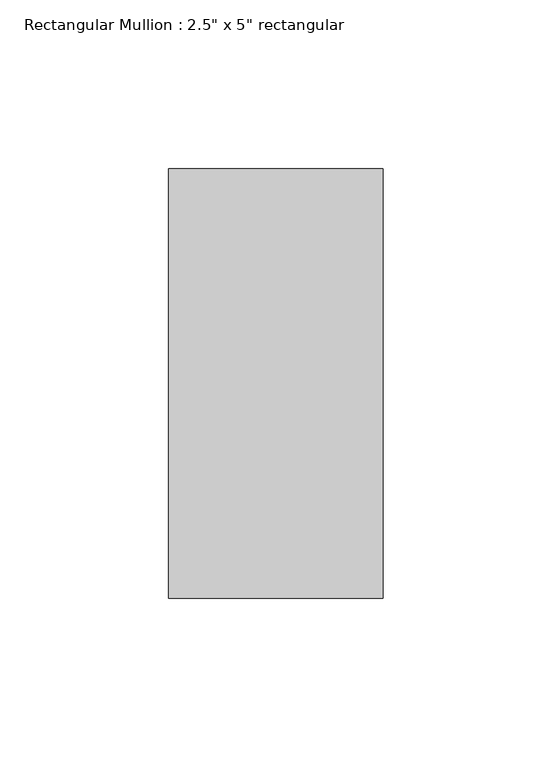
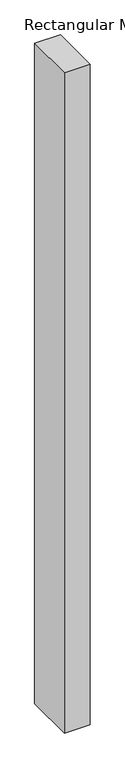
"""IFC4 building model written with IfcOpenShell, lengths in millimetres: member geometry."""

from ifc_helpers import new_model, si_unit, frame, origin, place, context, project, spatial, polyline, outline, extrude, source, transform, mapped, element, save


def member_4301f95b(model_context):
    return source(origin(), model_context, "Body", "SweptSolid", [
        extrude(outline(polyline([(0.0, 63.5), (0.0, -63.5), (-63.5, -63.5), (-63.5, 63.5), (0.0, 63.5)])), frame((0.0, 0.0, -1728.1374524), z_axis=(0.0, 0.0, 1.0), x_axis=(1.0, 0.0, 0.0)), (0.0, 0.0, 1.0), 1728.1374524),
    ])


if __name__ == "__main__":
    model = new_model("IFC4")
    model_context = context("Model", 3, world=origin())
    ifc_project = project(units=[si_unit("LENGTHUNIT", "METRE", prefix="MILLI")], contexts=[model_context])
    site = spatial("IfcSite", under=ifc_project)
    building = spatial("IfcBuilding", under=site)
    placement = place(None, origin())
    member_shape = member_4301f95b(model_context)
    element("IfcMember", 1, ObjectType="Rectangular Mullion : 2.5\" x 5\" rectangular", at=placement, inside=building, context=model_context, shape_type="MappedRepresentation", body=[
        mapped(member_shape, transform((0.0, 0.0, 0.0), x_axis=(1.0, 0.0, 0.0), y_axis=(0.0, 1.0, 0.0), z_axis=(0.0, 0.0, 1.0))),
    ])
    save(model, "model.ifc")

# Revit data of these elements
# Type "Rectangular Mullion : 2.5\" x 5\" rectangular"
#   built-in parameter 1007304 = 0.416667 (stored number, unit not read)
#   built-in parameter 1007301 = 0.104167 (stored number, unit not read)
#   built-in parameter 1007300 = 0.104167 (stored number, unit not read)
# Element 1 (IfcMember, "Rectangular Mullion : 2.5\" x 5\" rectangular")
#   Materials on its faces: "Aluminum"
# Materials
#   "Aluminum": class "Metal", colour RGB 247 247 247, transparency 0, Description = "Aluminum 6061", Cost = 0
